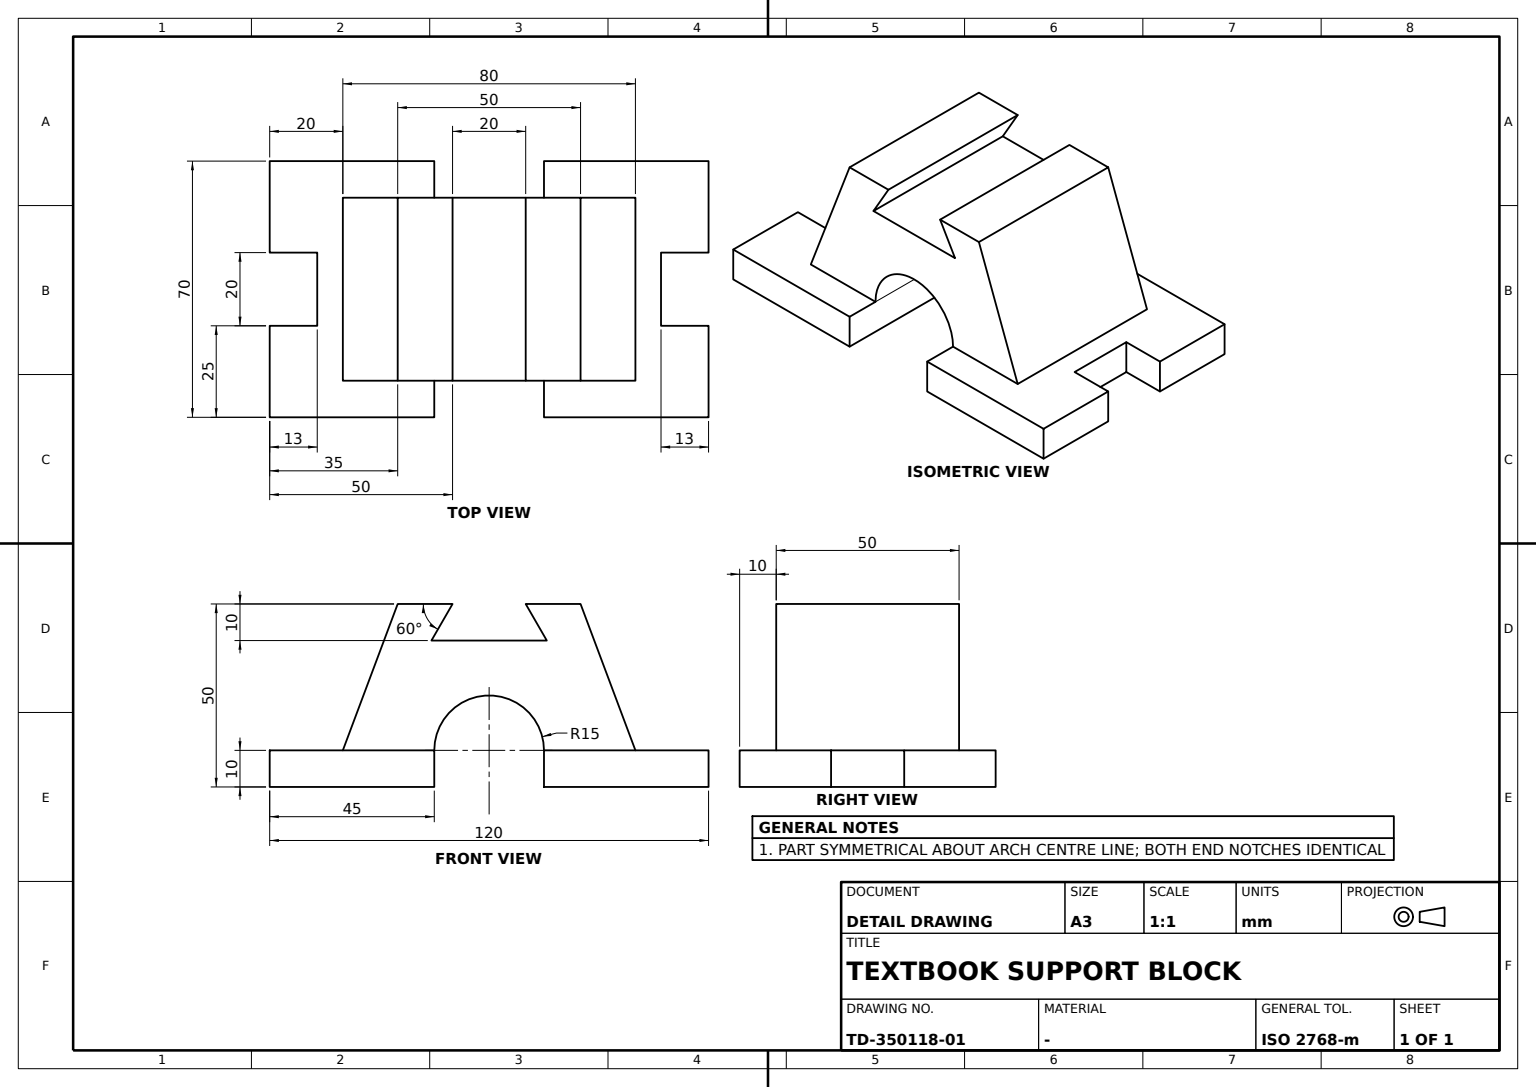
CATIA V5 part; units mm, degrees
sketch "Sketch1" plane through (0, 0, 0) normal (0, 0, 1) x (1, 0, 0)
  line L0 (60, 35) -> (60, -35)
  line L1 (60, -35) -> (-60, -35)
  line L2 (-60, -35) -> (-60, 35)
  line L3 (-60, 35) -> (60, 35)
  dimension "length L0" = 70
  dimension "length L1" = 120
  constraint vertical L0 y-axis
  constraint vertical L2 y-axis
  constraint horizontal L1 x-axis
  constraint horizontal L3 x-axis
  constraint equidistance L0 L2 origin
  constraint equidistance L1 L3 origin
extrude "Pad1" add sketch "Sketch1" along normal blind 10
sketch "Sketch2" plane through (0, 0, 0) normal (0, 1, 0) x (-1, 0, 0)
  line L0 (-25, 50) -> (25, 50)
  point P0 (0, 50)
  line L1 (-60, 10) -> (60, 10) construction
  line L2 (-40, 10) -> (40, 10)
  point P1 (0, 10)
  point P2 (40, 10)
  line L3 (-60, 0) -> (60, 0) construction
  line L4 (-25, 50) -> (-40, 10)
  line L5 (25, 50) -> (40, 10)
  point P3 (40, 10)
  dimension "length L0" = 50
  dimension "distance L0 L1" = 40
  dimension "length L2" = 80
  dimension "distance L2 L3" = 10
  constraint midpoint L0 P0
  constraint midpoint L2 P1
  constraint coincidence P0 y-axis
  constraint coincidence P1 y-axis
  constraint coincidence P3 L2
  constraint coincidence P3 P2
  constraint horizontal L0 x-axis
  constraint horizontal L2 x-axis
extrude "Pad2" add sketch "Sketch2" along normal mid plane 50
sketch "Sketch3" plane through (0, -35, 0) normal (0, -1, 0) x (1, 0, 0)
  line L0 (-15, 0) -> (15, 0)
  point P0 (15, 0)
  line L1 (15, 0) -> (15, 10)
  point P1 (15, 0)
  line L2 (-15, 0) -> (-15, 10)
  arc A0 (-15, 10) -> (15, 10) centre (0, 10) cw
  dimension "length L0" = 30
  dimension "length L1" = 10
  dimension "length L2" = 10
  constraint midpoint L0 origin
  constraint horizontal L0 x-axis
  constraint vertical L1 y-axis
  constraint vertical L2 y-axis
  constraint coincidence P1 P0
  constraint tangency A0 L1
extrude "Pocket1" cut sketch "Sketch3" against normal through all
sketch "Sketch4" plane through (0, -25, 0) normal (0, -1, 0) x (1, 0, 0)
  line L0 (-10, 50) -> (10, 50)
  point P0 (0, 50)
  point P1 (-10, 50)
  point P2 (10, 50)
  line L1 (-25, 50) -> (25, 50) construction
  line L2 (-10, 50) -> (-15.7735, 40)
  point P3 (-15.7735, 40)
  point P4 (15.7735, 40)
  point P5 (10, 50)
  line L3 (10, 50) -> (15.7735, 40)
  line L4 (-15.7735, 40) -> (15.7735, 40)
  dimension "length L0" = 20
  dimension "angle L2 x axis" = 60
  dimension "distance P3 L0" = 10
  constraint midpoint L0 P0
  constraint coincidence P0 y-axis
  constraint coincidence L0 L1
  constraint coincidence P2 P5
  constraint horizontal L0 x-axis
  constraint horizontal L4 x-axis
  constraint symmetry P3 P4 y-axis
  constraint symmetry P1 P5 y-axis
  constraint symmetry L2 L3 y-axis
extrude "Pocket2" cut sketch "Sketch4" against normal through all
sketch "Sketch5" plane through (0, 0, 10) normal (0, 0, 1) x (1, 0, 0)
  point P0 (53.5, 0)
  line L0 (60, 10) -> (60, -10)
  line L1 (60, -10) -> (47, -10)
  line L2 (47, -10) -> (47, 10)
  line L3 (47, 10) -> (60, 10)
  point P1 (60, 10)
  point P2 (60, -10)
  point P3 (47, -10)
  point P4 (47, 10)
  line L4 (60, -35) -> (60, 35) construction
  point P5 (-47, -10)
  point P6 (-60, -10)
  line L5 (-60, -10) -> (-47, -10)
  point P7 (-47, 10)
  line L6 (-47, -10) -> (-47, 10)
  point P8 (-60, 10)
  line L7 (-47, 10) -> (-60, 10)
  line L8 (-60, 10) -> (-60, -10)
  dimension "length L3" = 13
  dimension "length L0" = 20
  constraint coincidence P0 x-axis
  constraint coincidence L0 L4
  constraint vertical L0 y-axis
  constraint vertical L2 y-axis
  constraint horizontal L1 x-axis
  constraint horizontal L3 x-axis
  constraint equidistance L0 L2 P0
  constraint equidistance L1 L3 P0
  constraint symmetry P3 P5 y-axis
  constraint symmetry P2 P6 y-axis
  constraint symmetry L1 L5 y-axis
  constraint symmetry P4 P7 y-axis
  constraint symmetry L2 L6 y-axis
  constraint symmetry P1 P8 y-axis
  constraint symmetry L3 L7 y-axis
  constraint symmetry L0 L8 y-axis
extrude "Pocket3" cut sketch "Sketch5" against normal through all
